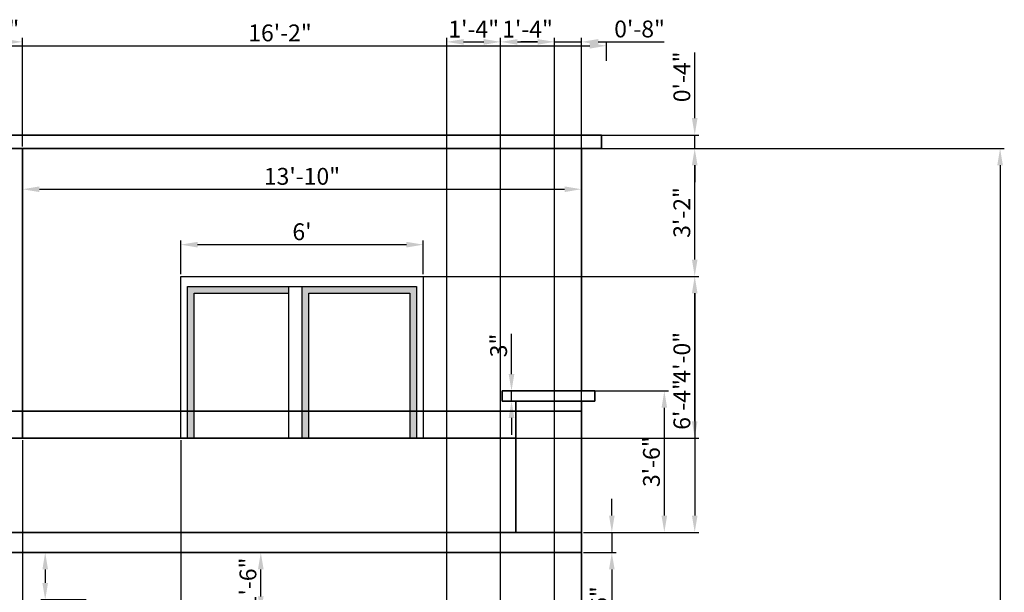
# Model space of a CAD drawing. Units: inches. Extents: x 2406 to 2953, y 1777 to 2285.
# Tile 5 of 5: x 2661 to 2953, y 2111 to 2281. Entities that reach past the tile are written whole.
import ezdxf

# ---------------------------------------------------------------- set-up
doc = ezdxf.new("R2010")
doc.units = ezdxf.units.IN
for name, color, linetype, lineweight in [('A-ANNO-DIMS', 2, 'Continuous', 18), ('A-DOOR', 3, 'Continuous', 25), ('A-ELEV', 7, 'Continuous', 35), ('A-ELEV-PATT', 253, 'Continuous', 13)]:
    doc.layers.add(name, color=color, linetype=linetype, lineweight=lineweight)
doc.styles.get("Standard").update_dxf_attribs({"font": 'arial.ttf'})
doc.dimstyles.new('ISO-25', dxfattribs={"dimtxt": 5, "dimasz": 5, "dimexe": 1.25, "dimexo": 0.625, "dimtad": 1, "dimdec": 0, "dimlunit": 3, "dimtxsty": 'Standard', "dimcen": 2.5, "dimadec": 0, "dimazin": 0, "dimtfac": 1, "dimtdec": 0, "dimtmove": 0, "dimatfit": 3, "dimfxl": 1, "dimarcsym": 0})

# ---------------------------------------------------------------- blocks, each defined once
blk = doc.blocks.new('*D1')
at = {"layer": 'A-ANNO-DIMS', "color": 0, "lineweight": -2, "transparency": 16777216}
for p, q in [((2828.46, 2242.34), (2953.44, 2242.34)), ((2952.19, 2237.34), (2952.19, 1827.34)), ((2828.46, 1822.34), (2953.44, 1822.34))]:
    blk.add_line(p, q, dxfattribs=at)
at = {"layer": 'A-ANNO-DIMS', "color": 0, "transparency": 16777216}
for points in [[(2951.35, 2237.34), (2953.02, 2237.34), (2952.19, 2242.34)], [(2951.35, 1827.34), (2953.02, 1827.34), (2952.19, 1822.34)]]:
    blk.add_solid(points, dxfattribs=at)
at = {"layer": 'Defpoints', "color": 0, "transparency": 16777216}
for p in [(2827.83, 2242.34), (2827.83, 1822.34), (2952.19, 1822.34)]:
    blk.add_point(p, dxfattribs=at)
at = {"layer": 'A-ANNO-DIMS', "color": 0, "transparency": 16777216, "insert": (2949.01, 2032.34), "char_height": 5, "attachment_point": 5, "rotation": 90}
blk.add_mtext("35'", dxfattribs=at)
blk = doc.blocks.new('*D10')
at = {"layer": 'A-ANNO-DIMS', "color": 0, "lineweight": -2, "transparency": 16777216}
for p, q in [((2641.3, 2268.37), (2641.3, 2274.08)), ((2646.3, 2272.83), (2830.3, 2272.83)), ((2835.3, 2268.37), (2835.3, 2274.08))]:
    blk.add_line(p, q, dxfattribs=at)
at = {"layer": 'A-ANNO-DIMS', "color": 0, "transparency": 16777216}
for points in [[(2646.3, 2273.66), (2646.3, 2272), (2641.3, 2272.83)], [(2830.3, 2273.66), (2830.3, 2272), (2835.3, 2272.83)]]:
    blk.add_solid(points, dxfattribs=at)
at = {"layer": 'Defpoints', "color": 0, "transparency": 16777216}
for p in [(2835.3, 2272.83), (2641.3, 2267.75), (2835.3, 2267.75)]:
    blk.add_point(p, dxfattribs=at)
at = {"layer": 'A-ANNO-DIMS', "color": 0, "transparency": 16777216, "insert": (2738.3, 2276.01), "char_height": 5, "attachment_point": 5}
blk.add_mtext('16\'-2"', dxfattribs=at)
blk = doc.blocks.new('*D11')
at = {"layer": 'A-ANNO-DIMS', "color": 0, "lineweight": -2, "transparency": 16777216}
for p, q in [((2708.83, 2204.97), (2708.83, 2215.03)), ((2780.83, 2204.97), (2780.83, 2215.03)), ((2713.83, 2213.78), (2775.83, 2213.78))]:
    blk.add_line(p, q, dxfattribs=at)
at = {"layer": 'A-ANNO-DIMS', "color": 0, "transparency": 16777216}
for points in [[(2713.83, 2214.61), (2713.83, 2212.94), (2708.83, 2213.78)], [(2775.83, 2214.61), (2775.83, 2212.94), (2780.83, 2213.78)]]:
    blk.add_solid(points, dxfattribs=at)
at = {"layer": 'Defpoints', "color": 0, "transparency": 16777216}
for p in [(2780.83, 2213.78), (2708.83, 2204.34), (2780.83, 2204.34)]:
    blk.add_point(p, dxfattribs=at)
at = {"layer": 'A-ANNO-DIMS', "color": 0, "transparency": 16777216, "insert": (2744.83, 2216.96), "char_height": 5, "attachment_point": 5}
blk.add_mtext("6'", dxfattribs=at)
blk = doc.blocks.new('*D12')
at = {"layer": 'A-ANNO-DIMS', "color": 0, "lineweight": -2, "transparency": 16777216}
for p, q in [((2661.83, 2241.72), (2661.83, 2228.99)), ((2827.83, 2241.72), (2827.83, 2228.99)), ((2666.83, 2230.24), (2822.83, 2230.24))]:
    blk.add_line(p, q, dxfattribs=at)
at = {"layer": 'A-ANNO-DIMS', "color": 0, "transparency": 16777216}
for points in [[(2666.83, 2231.07), (2666.83, 2229.4), (2661.83, 2230.24)], [(2822.83, 2231.07), (2822.83, 2229.4), (2827.83, 2230.24)]]:
    blk.add_solid(points, dxfattribs=at)
at = {"layer": 'Defpoints', "color": 0, "transparency": 16777216}
for p in [(2661.83, 2242.34), (2827.83, 2242.34), (2827.83, 2230.24)]:
    blk.add_point(p, dxfattribs=at)
at = {"layer": 'A-ANNO-DIMS', "color": 0, "transparency": 16777216, "insert": (2744.83, 2233.42), "char_height": 5, "attachment_point": 5}
blk.add_mtext('13\'-10"', dxfattribs=at)
blk = doc.blocks.new('*D26')
at = {"layer": 'A-ANNO-DIMS', "color": 0, "lineweight": -2, "transparency": 16777216}
for p, q in [((2680.71, 2122.34), (2667.31, 2122.34)), ((2668.56, 2117.34), (2668.56, 2113.34)), ((2680.71, 2108.34), (2667.31, 2108.34)), ((2668.56, 2108.34), (2668.56, 2089.27))]:
    blk.add_line(p, q, dxfattribs=at)
at = {"layer": 'A-ANNO-DIMS', "color": 0, "transparency": 16777216}
for points in [[(2667.73, 2117.34), (2669.4, 2117.34), (2668.56, 2122.34)], [(2667.73, 2113.34), (2669.4, 2113.34), (2668.56, 2108.34)]]:
    blk.add_solid(points, dxfattribs=at)
at = {"layer": 'Defpoints', "color": 0, "transparency": 16777216}
for p in [(2681.33, 2122.34), (2668.56, 2108.34), (2681.33, 2108.34)]:
    blk.add_point(p, dxfattribs=at)
at = {"layer": 'A-ANNO-DIMS', "color": 0, "transparency": 16777216, "insert": (2665.43, 2096.31), "char_height": 5, "attachment_point": 5, "rotation": 90}
blk.add_mtext('1\'-2"', dxfattribs=at)
blk = doc.blocks.new('*D27')
at = {"layer": 'A-ANNO-DIMS', "color": 0, "lineweight": -2, "transparency": 16777216}
for p, q in [((2737.53, 2122.34), (2731.35, 2122.34)), ((2732.6, 2109.34), (2732.6, 2117.34)), ((2737.53, 2104.34), (2731.35, 2104.34))]:
    blk.add_line(p, q, dxfattribs=at)
at = {"layer": 'A-ANNO-DIMS', "color": 0, "transparency": 16777216}
for points in [[(2731.77, 2117.34), (2733.44, 2117.34), (2732.6, 2122.34)], [(2731.77, 2109.34), (2733.44, 2109.34), (2732.6, 2104.34)]]:
    blk.add_solid(points, dxfattribs=at)
at = {"layer": 'Defpoints', "color": 0, "transparency": 16777216}
for p in [(2732.6, 2122.34), (2738.16, 2122.34), (2738.16, 2104.34)]:
    blk.add_point(p, dxfattribs=at)
at = {"layer": 'A-ANNO-DIMS', "color": 0, "transparency": 16777216, "insert": (2729.43, 2113.34), "char_height": 5, "attachment_point": 5, "rotation": 90}
blk.add_mtext('1\'-6"', dxfattribs=at)
blk = doc.blocks.new('*D28')
at = {"layer": 'A-ANNO-DIMS', "color": 0, "lineweight": -2, "transparency": 16777216}
for p, q in [((2828.46, 2170.34), (2853.71, 2170.34)), ((2852.46, 2133.34), (2852.46, 2165.34)), ((2828.46, 2128.34), (2853.71, 2128.34))]:
    blk.add_line(p, q, dxfattribs=at)
at = {"layer": 'A-ANNO-DIMS', "color": 0, "transparency": 16777216}
for points in [[(2851.62, 2165.34), (2853.29, 2165.34), (2852.46, 2170.34)], [(2851.62, 2133.34), (2853.29, 2133.34), (2852.46, 2128.34)]]:
    blk.add_solid(points, dxfattribs=at)
at = {"layer": 'Defpoints', "color": 0, "transparency": 16777216}
for p in [(2827.83, 2170.34), (2852.46, 2170.34), (2827.83, 2128.34)]:
    blk.add_point(p, dxfattribs=at)
at = {"layer": 'A-ANNO-DIMS', "color": 0, "transparency": 16777216, "insert": (2849.28, 2149.34), "char_height": 5, "attachment_point": 5, "rotation": 90}
blk.add_mtext('3\'-6"', dxfattribs=at)
blk = doc.blocks.new('*D29')
at = {"layer": 'A-ANNO-DIMS', "color": 0, "lineweight": -2, "transparency": 16777216}
for p, q in [((2836.87, 2133.34), (2836.87, 2138.34)), ((2828.46, 2128.34), (2838.12, 2128.34)), ((2836.87, 2128.34), (2836.87, 2122.34)), ((2828.46, 2122.34), (2838.12, 2122.34)), ((2836.87, 2117.34), (2836.87, 2105.32))]:
    blk.add_line(p, q, dxfattribs=at)
at = {"layer": 'A-ANNO-DIMS', "color": 0, "transparency": 16777216}
for points in [[(2836.03, 2133.34), (2837.7, 2133.34), (2836.87, 2128.34)], [(2836.03, 2117.34), (2837.7, 2117.34), (2836.87, 2122.34)]]:
    blk.add_solid(points, dxfattribs=at)
at = {"layer": 'Defpoints', "color": 0, "transparency": 16777216}
for p in [(2827.83, 2128.34), (2827.83, 2122.34), (2836.87, 2122.34)]:
    blk.add_point(p, dxfattribs=at)
at = {"layer": 'A-ANNO-DIMS', "color": 0, "transparency": 16777216, "insert": (2833.69, 2108.83), "char_height": 5, "attachment_point": 5, "rotation": 90}
blk.add_mtext('6"', dxfattribs=at)
blk = doc.blocks.new('*D37')
at = {"layer": 'A-ANNO-DIMS', "color": 0, "lineweight": -2, "transparency": 16777216}
for p, q in [((2807.06, 2175.34), (2807.06, 2187.33)), ((2804.93, 2170.34), (2808.31, 2170.34)), ((2807.06, 2167.34), (2807.06, 2170.34)), ((2804.93, 2167.34), (2808.31, 2167.34)), ((2807.06, 2162.34), (2807.06, 2157.34))]:
    blk.add_line(p, q, dxfattribs=at)
at = {"layer": 'A-ANNO-DIMS', "color": 0, "transparency": 16777216}
for points in [[(2806.23, 2175.34), (2807.9, 2175.34), (2807.06, 2170.34)], [(2806.23, 2162.34), (2807.9, 2162.34), (2807.06, 2167.34)]]:
    blk.add_solid(points, dxfattribs=at)
at = {"layer": 'Defpoints', "color": 0, "transparency": 16777216}
for p in [(2804.31, 2170.34), (2807.06, 2170.34), (2804.31, 2167.34)]:
    blk.add_point(p, dxfattribs=at)
at = {"layer": 'A-ANNO-DIMS', "color": 0, "transparency": 16777216, "insert": (2803.88, 2183.84), "char_height": 5, "attachment_point": 5, "rotation": 90}
blk.add_mtext('3"', dxfattribs=at)
blk = doc.blocks.new('*D51')
at = {"layer": 'A-ANNO-DIMS', "color": 0, "lineweight": -2, "transparency": 16777216}
for p, q in [((2787.83, 1984.97), (2787.83, 2275.24)), ((2792.83, 2273.99), (2798.83, 2273.99)), ((2803.83, 1984.97), (2803.83, 2275.24))]:
    blk.add_line(p, q, dxfattribs=at)
at = {"layer": 'A-ANNO-DIMS', "color": 0, "transparency": 16777216}
for points in [[(2792.83, 2274.82), (2792.83, 2273.16), (2787.83, 2273.99)], [(2798.83, 2274.82), (2798.83, 2273.16), (2803.83, 2273.99)]]:
    blk.add_solid(points, dxfattribs=at)
at = {"layer": 'Defpoints', "color": 0, "transparency": 16777216}
for p in [(2803.83, 2273.99), (2787.83, 1984.34), (2803.83, 1984.34)]:
    blk.add_point(p, dxfattribs=at)
at = {"layer": 'A-ANNO-DIMS', "color": 0, "transparency": 16777216, "insert": (2795.83, 2277.13), "char_height": 5, "attachment_point": 5}
blk.add_mtext('1\'-4"', dxfattribs=at)
blk = doc.blocks.new('*D52')
at = {"layer": 'A-ANNO-DIMS', "color": 0, "lineweight": -2, "transparency": 16777216}
for p, q in [((2803.83, 1984.97), (2803.83, 2275.24)), ((2808.83, 2273.99), (2814.83, 2273.99)), ((2819.83, 1984.97), (2819.83, 2275.24))]:
    blk.add_line(p, q, dxfattribs=at)
at = {"layer": 'A-ANNO-DIMS', "color": 0, "transparency": 16777216}
for points in [[(2808.83, 2274.82), (2808.83, 2273.16), (2803.83, 2273.99)], [(2814.83, 2274.82), (2814.83, 2273.16), (2819.83, 2273.99)]]:
    blk.add_solid(points, dxfattribs=at)
at = {"layer": 'Defpoints', "color": 0, "transparency": 16777216}
for p in [(2819.83, 2273.99), (2803.83, 1984.34), (2819.83, 1984.34)]:
    blk.add_point(p, dxfattribs=at)
at = {"layer": 'A-ANNO-DIMS', "color": 0, "transparency": 16777216, "insert": (2811.83, 2277.13), "char_height": 5, "attachment_point": 5}
blk.add_mtext('1\'-4"', dxfattribs=at)
blk = doc.blocks.new('*D53')
at = {"layer": 'A-ANNO-DIMS', "color": 0, "lineweight": -2, "transparency": 16777216}
for p, q in [((2814.83, 2273.99), (2809.83, 2273.99)), ((2819.83, 1984.97), (2819.83, 2275.24)), ((2819.83, 2273.99), (2827.83, 2273.99)), ((2827.83, 1984.97), (2827.83, 2275.24)), ((2832.83, 2273.99), (2852.37, 2273.99))]:
    blk.add_line(p, q, dxfattribs=at)
at = {"layer": 'A-ANNO-DIMS', "color": 0, "transparency": 16777216}
for points in [[(2814.83, 2274.82), (2814.83, 2273.16), (2819.83, 2273.99)], [(2832.83, 2274.82), (2832.83, 2273.16), (2827.83, 2273.99)]]:
    blk.add_solid(points, dxfattribs=at)
at = {"layer": 'Defpoints', "color": 0, "transparency": 16777216}
for p in [(2827.83, 2273.99), (2819.83, 1984.34), (2827.83, 1984.34)]:
    blk.add_point(p, dxfattribs=at)
at = {"layer": 'A-ANNO-DIMS', "color": 0, "transparency": 16777216, "insert": (2845.1, 2277.17), "char_height": 5, "attachment_point": 5}
blk.add_mtext('0\'-8"', dxfattribs=at)
blk = doc.blocks.new('*D79')
at = {"layer": 'A-ANNO-DIMS', "color": 0, "lineweight": -2, "transparency": 16777216}
for p, q in [((2861.48, 2251.34), (2861.48, 2270.88)), ((2640.46, 2246.34), (2862.73, 2246.34)), ((2861.48, 2242.34), (2861.48, 2246.34)), ((2640.46, 2242.34), (2862.73, 2242.34)), ((2861.48, 2237.34), (2861.48, 2232.34))]:
    blk.add_line(p, q, dxfattribs=at)
at = {"layer": 'A-ANNO-DIMS', "color": 0, "transparency": 16777216}
for points in [[(2860.65, 2251.34), (2862.32, 2251.34), (2861.48, 2246.34)], [(2860.65, 2237.34), (2862.32, 2237.34), (2861.48, 2242.34)]]:
    blk.add_solid(points, dxfattribs=at)
at = {"layer": 'Defpoints', "color": 0, "transparency": 16777216}
for p in [(2639.83, 2246.34), (2861.48, 2246.34), (2639.83, 2242.34)]:
    blk.add_point(p, dxfattribs=at)
at = {"layer": 'A-ANNO-DIMS', "color": 0, "transparency": 16777216, "insert": (2858.31, 2263.61), "char_height": 5, "attachment_point": 5, "rotation": 90}
blk.add_mtext('0\'-4"', dxfattribs=at)
blk = doc.blocks.new('*D80')
at = {"layer": 'A-ANNO-DIMS', "color": 0, "lineweight": -2, "transparency": 16777216}
for p, q in [((2644.83, 2242.97), (2644.83, 2275.24)), ((2649.83, 2273.99), (2656.83, 2273.99)), ((2661.83, 2242.97), (2661.83, 2275.24))]:
    blk.add_line(p, q, dxfattribs=at)
at = {"layer": 'A-ANNO-DIMS', "color": 0, "transparency": 16777216}
for points in [[(2649.83, 2274.82), (2649.83, 2273.16), (2644.83, 2273.99)], [(2656.83, 2274.82), (2656.83, 2273.16), (2661.83, 2273.99)]]:
    blk.add_solid(points, dxfattribs=at)
at = {"layer": 'Defpoints', "color": 0, "transparency": 16777216}
for p in [(2661.83, 2273.99), (2644.83, 2242.34), (2661.83, 2242.34)]:
    blk.add_point(p, dxfattribs=at)
at = {"layer": 'A-ANNO-DIMS', "color": 0, "transparency": 16777216, "insert": (2653.33, 2277.17), "char_height": 5, "attachment_point": 5}
blk.add_mtext('1\'-5"', dxfattribs=at)
blk = doc.blocks.new('*D81')
at = {"layer": 'A-ANNO-DIMS', "color": 0, "lineweight": -2, "transparency": 16777216}
for p, q in [((2709.46, 2204.34), (2862.73, 2204.34)), ((2861.48, 2161.34), (2861.48, 2199.34)), ((2709.46, 2156.34), (2862.73, 2156.34))]:
    blk.add_line(p, q, dxfattribs=at)
at = {"layer": 'A-ANNO-DIMS', "color": 0, "transparency": 16777216}
for points in [[(2860.65, 2199.34), (2862.32, 2199.34), (2861.48, 2204.34)], [(2860.65, 2161.34), (2862.32, 2161.34), (2861.48, 2156.34)]]:
    blk.add_solid(points, dxfattribs=at)
at = {"layer": 'Defpoints', "color": 0, "transparency": 16777216}
for p in [(2708.83, 2204.34), (2861.48, 2204.34), (2708.83, 2156.34)]:
    blk.add_point(p, dxfattribs=at)
at = {"layer": 'A-ANNO-DIMS', "color": 0, "transparency": 16777216, "insert": (2858.31, 2180.34), "char_height": 5, "attachment_point": 5, "rotation": 90}
blk.add_mtext('4\'-0"', dxfattribs=at)
blk = doc.blocks.new('*D82')
at = {"layer": 'A-ANNO-DIMS', "color": 0, "lineweight": -2, "transparency": 16777216}
for p, q in [((2661.83, 2155.72), (2661.83, 1793.44)), ((2708.83, 2155.72), (2708.83, 1793.44)), ((2666.83, 1794.69), (2703.83, 1794.69))]:
    blk.add_line(p, q, dxfattribs=at)
at = {"layer": 'A-ANNO-DIMS', "color": 0, "transparency": 16777216}
for points in [[(2666.83, 1795.52), (2666.83, 1793.86), (2661.83, 1794.69)], [(2703.83, 1795.52), (2703.83, 1793.86), (2708.83, 1794.69)]]:
    blk.add_solid(points, dxfattribs=at)
at = {"layer": 'Defpoints', "color": 0, "transparency": 16777216}
for p in [(2661.83, 2156.34), (2708.83, 2156.34), (2708.83, 1794.69)]:
    blk.add_point(p, dxfattribs=at)
at = {"layer": 'A-ANNO-DIMS', "color": 0, "transparency": 16777216, "insert": (2685.33, 1797.87), "char_height": 5, "attachment_point": 5}
blk.add_mtext('3\'-11"', dxfattribs=at)
blk = doc.blocks.new('*D83')
at = {"layer": 'A-ANNO-DIMS', "color": 0, "lineweight": -2, "transparency": 16777216}
for p, q in [((2828.46, 2242.34), (2862.73, 2242.34)), ((2861.48, 2209.34), (2861.48, 2237.34)), ((2781.46, 2204.34), (2862.73, 2204.34))]:
    blk.add_line(p, q, dxfattribs=at)
at = {"layer": 'A-ANNO-DIMS', "color": 0, "transparency": 16777216}
for points in [[(2860.65, 2237.34), (2862.32, 2237.34), (2861.48, 2242.34)], [(2860.65, 2209.34), (2862.32, 2209.34), (2861.48, 2204.34)]]:
    blk.add_solid(points, dxfattribs=at)
at = {"layer": 'Defpoints', "color": 0, "transparency": 16777216}
for p in [(2827.83, 2242.34), (2861.48, 2242.34), (2780.83, 2204.34)]:
    blk.add_point(p, dxfattribs=at)
at = {"layer": 'A-ANNO-DIMS', "color": 0, "transparency": 16777216, "insert": (2858.3, 2223.34), "char_height": 5, "attachment_point": 5, "rotation": 90}
blk.add_mtext('3\'-2"', dxfattribs=at)
blk = doc.blocks.new('*D84')
at = {"layer": 'A-ANNO-DIMS', "color": 0, "lineweight": -2, "transparency": 16777216}
for p, q in [((2781.46, 2204.34), (2862.73, 2204.34)), ((2861.48, 2199.34), (2861.48, 2133.34)), ((2828.46, 2128.34), (2862.73, 2128.34))]:
    blk.add_line(p, q, dxfattribs=at)
at = {"layer": 'A-ANNO-DIMS', "color": 0, "transparency": 16777216}
for points in [[(2860.65, 2199.34), (2862.32, 2199.34), (2861.48, 2204.34)], [(2860.65, 2133.34), (2862.32, 2133.34), (2861.48, 2128.34)]]:
    blk.add_solid(points, dxfattribs=at)
at = {"layer": 'Defpoints', "color": 0, "transparency": 16777216}
for p in [(2780.83, 2204.34), (2827.83, 2128.34), (2861.48, 2128.34)]:
    blk.add_point(p, dxfattribs=at)
at = {"layer": 'A-ANNO-DIMS', "color": 0, "transparency": 16777216, "insert": (2858.31, 2166.34), "char_height": 5, "attachment_point": 5, "rotation": 90}
blk.add_mtext('6\'-4"', dxfattribs=at)

msp = doc.modelspace()

# ---------------------------------------------------------------- hatches: boundary and pattern name
at = {"layer": 'A-ELEV-PATT'}
h = msp.add_hatch(color=256, dxfattribs=at)
h.dxf.hatch_style = 1
h.paths.add_polyline_path([(2740.83, 2199.34), (2740.83, 2201.34), (2710.83, 2201.34), (2710.83, 2156.34), (2712.83, 2156.34), (2712.83, 2199.34)])
h = msp.add_hatch(color=256, dxfattribs=at)
h.dxf.hatch_style = 1
h.paths.add_polyline_path([(2776.83, 2199.34), (2776.83, 2156.34), (2778.83, 2156.34), (2778.83, 2201.34), (2744.83, 2201.34), (2744.83, 2156.34), (2746.83, 2156.34), (2746.83, 2199.34)])

# ---------------------------------------------------------------- linework, layer by layer
at = {"layer": 'A-DOOR'}
for p, q in [((2740.83, 2201.34), (2740.83, 2156.34)), ((2744.83, 2201.34), (2744.83, 2156.34))]:
    msp.add_line(p, q, dxfattribs=at)
for points in [[(2708.83, 2156.34), (2708.83, 2204.34), (2780.83, 2204.34), (2780.83, 2156.34)], [(2710.83, 2156.34), (2710.83, 2201.34), (2778.83, 2201.34), (2778.83, 2156.34)], [(2712.83, 2156.34), (2712.83, 2199.34), (2740.83, 2199.34)], [(2746.83, 2156.34), (2746.83, 2199.34), (2776.83, 2199.34), (2776.83, 2156.34)]]:
    msp.add_lwpolyline(points, dxfattribs=at)
at = {"layer": 'A-ELEV'}
for p, q in [((2833.83, 2246.34), (2639.83, 2246.34)), ((2833.83, 2242.34), (2833.83, 2246.34)), ((2833.83, 2242.34), (2639.83, 2242.34)), ((2827.83, 2242.34), (2661.83, 2242.34)), ((2661.83, 2222.34), (2661.83, 2242.34)), ((2827.83, 2170.34), (2827.83, 2242.34)), ((2827.83, 2170.34), (2827.83, 2242.34)), ((2827.83, 2222.34), (2827.83, 2242.34)), ((2827.83, 2222.34), (2827.83, 2242.34)), ((2661.83, 2156.34), (2661.83, 2222.34)), ((2831.83, 2170.34), (2804.31, 2170.34)), ((2804.31, 2167.34), (2804.31, 2170.34)), ((2831.83, 2167.34), (2831.83, 2170.34)), ((2831.83, 2167.34), (2804.31, 2167.34)), ((2808.31, 2128.34), (2808.31, 2167.34)), ((2827.83, 1822.34), (2827.83, 2167.34)), ((2635.33, 2164.34), (2827.83, 2164.34)), ((2635.33, 2156.34), (2808.31, 2156.34)), ((2661.83, 2156.34), (2808.31, 2156.34)), ((2443.83, 2128.34), (2827.83, 2128.34)), ((2443.83, 2122.34), (2827.83, 2122.34))]:
    msp.add_line(p, q, dxfattribs=at)

# ---------------------------------------------------------------- dimensions: what is measured, and where the dimension line sits
at = {"layer": 'A-ANNO-DIMS'}
for base, p1, p2, override, picture, middle in [((2835.3, 2272.83), (2641.3, 2267.75), (2835.3, 2267.75), {"dimclrd": 0, "dimclre": 0, "dimclrt": 0}, '*D10', (2738.3, 2276.01)), ((2661.83, 2273.99), (2644.83, 2242.34), (2661.83, 2242.34), {"dimdec": 1, "dimlfac": 1, "dimrnd": 0, "dimzin": 1, "dimdsep": 46, "dimlunit": 4, "dimfrac": 2}, '*D80', (2653.33, 2277.17)), ((2803.83, 2273.99), (2787.83, 1984.34), (2803.83, 1984.34), {"dimdec": 1, "dimlfac": 1, "dimrnd": 0, "dimzin": 1, "dimdsep": 46, "dimlunit": 4, "dimfrac": 2}, '*D51', (2795.83, 2277.13)), ((2819.83, 2273.99), (2803.83, 1984.34), (2819.83, 1984.34), {"dimdec": 1, "dimlfac": 1, "dimrnd": 0, "dimzin": 1, "dimdsep": 46, "dimlunit": 4, "dimfrac": 2}, '*D52', (2811.83, 2277.13)), ((2827.83, 2273.99), (2819.83, 1984.34), (2827.83, 1984.34), {"dimdec": 1, "dimlfac": 1, "dimrnd": 0, "dimzin": 1, "dimdsep": 46, "dimlunit": 4, "dimfrac": 2}, '*D53', (2845.1, 2277.17)), ((2827.83, 2230.24), (2661.83, 2242.34), (2827.83, 2242.34), {"dimclrd": 0, "dimclre": 0, "dimclrt": 0}, '*D12', (2744.83, 2233.42)), ((2780.83, 2213.78), (2708.83, 2204.34), (2780.83, 2204.34), {"dimclrd": 0, "dimclre": 0, "dimclrt": 0}, '*D11', (2744.83, 2216.96)), ((2708.83, 1794.69), (2661.83, 2156.34), (2708.83, 2156.34), {"dimdec": 1, "dimlfac": 1, "dimrnd": 0, "dimzin": 1, "dimdsep": 46, "dimlunit": 4, "dimfrac": 2}, '*D82', (2685.33, 1797.87))]:
    dim = msp.add_linear_dim(base=base, p1=p1, p2=p2, dimstyle='ISO-25', override=override, dxfattribs=at)
    dim.commit()
    dim.dimension.update_dxf_attribs({"geometry": picture, "text_midpoint": middle})
for base, p1, p2, override, picture, middle in [((2861.48, 2246.34), (2639.83, 2242.34), (2639.83, 2246.34), {"dimdec": 1, "dimlfac": 1, "dimrnd": 0, "dimzin": 1, "dimdsep": 46, "dimlunit": 4, "dimfrac": 2}, '*D79', (2858.31, 2263.61)), ((2861.48, 2242.34), (2780.83, 2204.34), (2827.83, 2242.34), {"dimdec": 1, "dimlfac": 1, "dimrnd": 0, "dimzin": 1, "dimdsep": 46, "dimlunit": 4, "dimfrac": 2}, '*D83', (2858.3, 2223.34)), ((2952.19, 1822.34), (2827.83, 2242.34), (2827.83, 1822.34), {"dimclrd": 0, "dimclre": 0, "dimclrt": 0}, '*D1', (2949.01, 2032.34)), ((2861.48, 2204.34), (2708.83, 2156.34), (2708.83, 2204.34), {"dimdec": 1, "dimlfac": 1, "dimrnd": 0, "dimzin": 1, "dimdsep": 46, "dimlunit": 4, "dimfrac": 2}, '*D81', (2858.31, 2180.34)), ((2861.48, 2128.34), (2780.83, 2204.34), (2827.83, 2128.34), {"dimdec": 1, "dimlfac": 1, "dimrnd": 0, "dimzin": 1, "dimdsep": 46, "dimlunit": 4, "dimfrac": 2}, '*D84', (2858.31, 2166.34)), ((2807.06, 2170.34), (2804.31, 2167.34), (2804.31, 2170.34), {"dimclrd": 0, "dimclre": 0, "dimclrt": 0}, '*D37', (2803.88, 2183.84)), ((2852.46, 2170.34), (2827.83, 2128.34), (2827.83, 2170.34), {"dimclrd": 0, "dimclre": 0, "dimclrt": 0}, '*D28', (2849.28, 2149.34)), ((2836.87, 2122.34), (2827.83, 2128.34), (2827.83, 2122.34), {"dimclrd": 0, "dimclre": 0, "dimclrt": 0}, '*D29', (2833.69, 2108.83)), ((2668.56, 2108.34), (2681.33, 2122.34), (2681.33, 2108.34), {"dimclrd": 0, "dimclre": 0, "dimclrt": 0}, '*D26', (2665.43, 2096.31)), ((2732.6, 2122.34), (2738.16, 2104.34), (2738.16, 2122.34), {"dimclrd": 0, "dimclre": 0, "dimclrt": 0}, '*D27', (2729.43, 2113.34))]:
    dim = msp.add_linear_dim(base=base, p1=p1, p2=p2, angle=90, dimstyle='ISO-25', override=override, dxfattribs=at)
    dim.commit()
    dim.dimension.update_dxf_attribs({"geometry": picture, "text_midpoint": middle})

doc.saveas('drawing.dxf')
